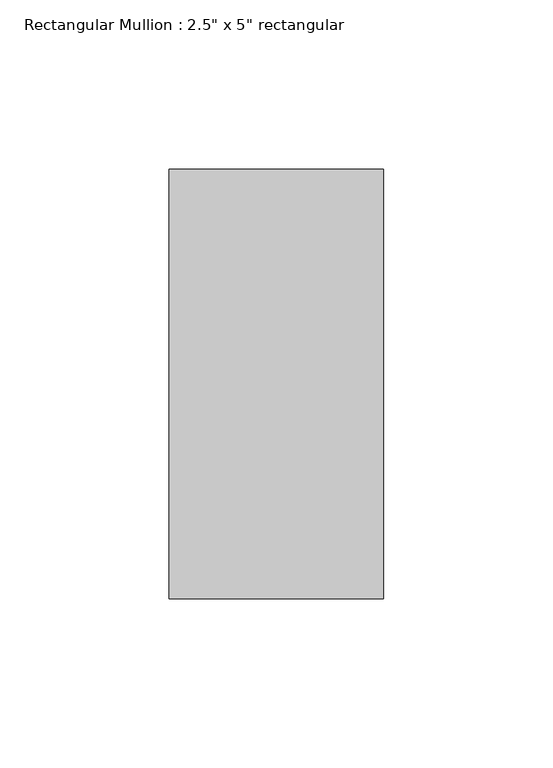
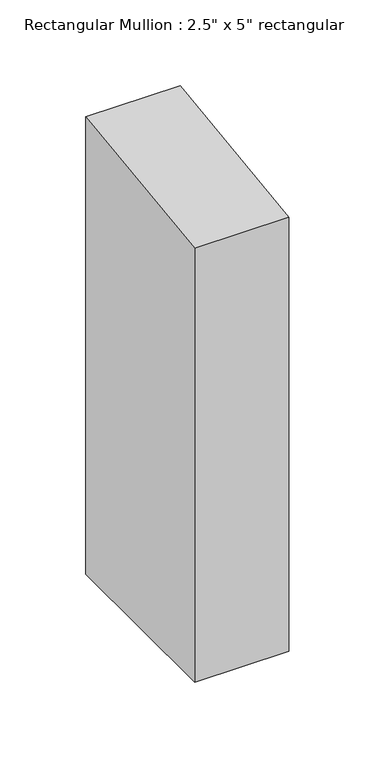
"""IFC4 building model written with IfcOpenShell, lengths in millimetres: member geometry."""

from ifc_helpers import new_model, si_unit, frame, origin, place, context, project, spatial, polyline, outline, extrude, source, transform, mapped, element, save


def member_d18c953d(model_context):
    return source(origin(), model_context, "Body", "SweptSolid", [
        extrude(outline(polyline([(-63.5, -8.2335242), (63.5, 8.2335242), (63.5, -317.1206388), (-63.5, -317.1206388), (-63.5, -8.2335242)])), frame((-63.5, 0.0, 0.0), z_axis=(1.0, 0.0, 0.0), x_axis=(0.0, 1.0, 0.0)), (0.0, 0.0, 1.0), 63.5),
    ])


if __name__ == "__main__":
    model = new_model("IFC4")
    model_context = context("Model", 3, world=origin())
    ifc_project = project(units=[si_unit("LENGTHUNIT", "METRE", prefix="MILLI")], contexts=[model_context])
    site = spatial("IfcSite", under=ifc_project)
    building = spatial("IfcBuilding", under=site)
    placement = place(None, origin())
    member_shape = member_d18c953d(model_context)
    element("IfcMember", 1, ObjectType="Rectangular Mullion : 2.5\" x 5\" rectangular", at=placement, inside=building, context=model_context, shape_type="MappedRepresentation", body=[
        mapped(member_shape, transform((0.0, 0.0, 0.0), x_axis=(1.0, 0.0, 0.0), y_axis=(0.0, 1.0, 0.0), z_axis=(0.0, 0.0, 1.0))),
    ])
    save(model, "model.ifc")

# Revit data of these elements
# Type "Rectangular Mullion : 2.5\" x 5\" rectangular"
#   built-in parameter 1007304 = 0.416667 (stored number, unit not read)
#   built-in parameter 1007301 = 0.104167 (stored number, unit not read)
#   built-in parameter 1007300 = 0.104167 (stored number, unit not read)
# Element 1 (IfcMember, "Rectangular Mullion : 2.5\" x 5\" rectangular")
#   Materials on its faces: "Iron, Ductile"
# Materials
#   "Iron, Ductile": class "Metal", colour RGB 0 0 0, transparency 0, Description = "Ductile cast iron", Cost = 0
